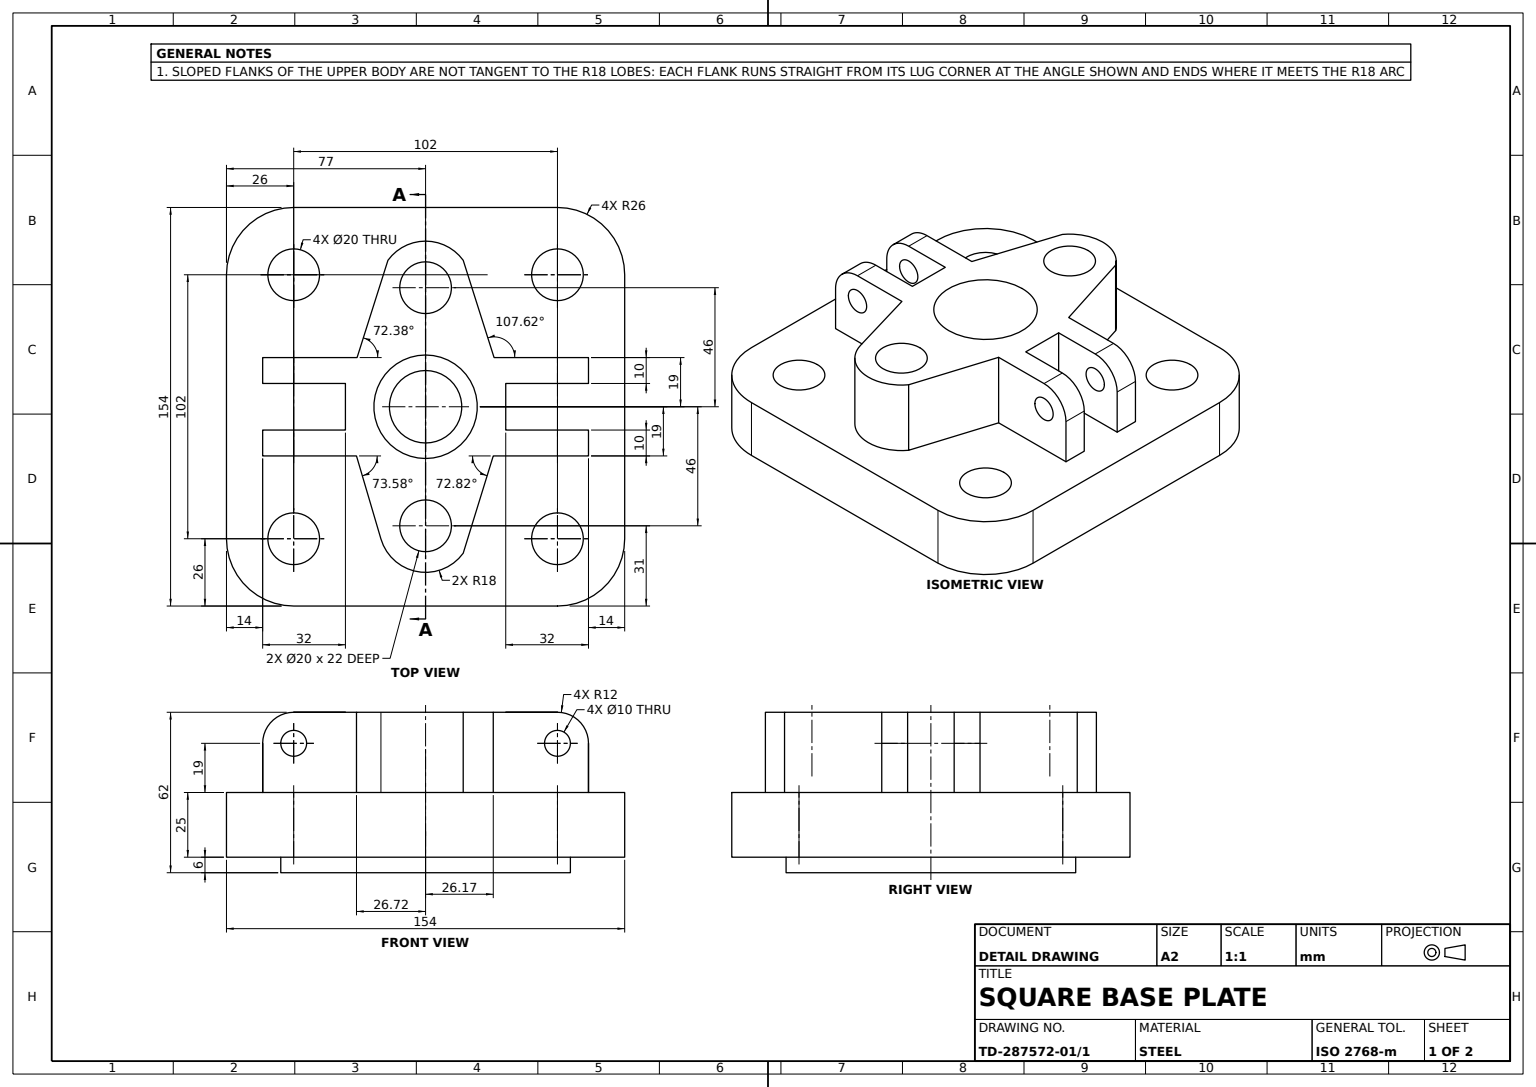
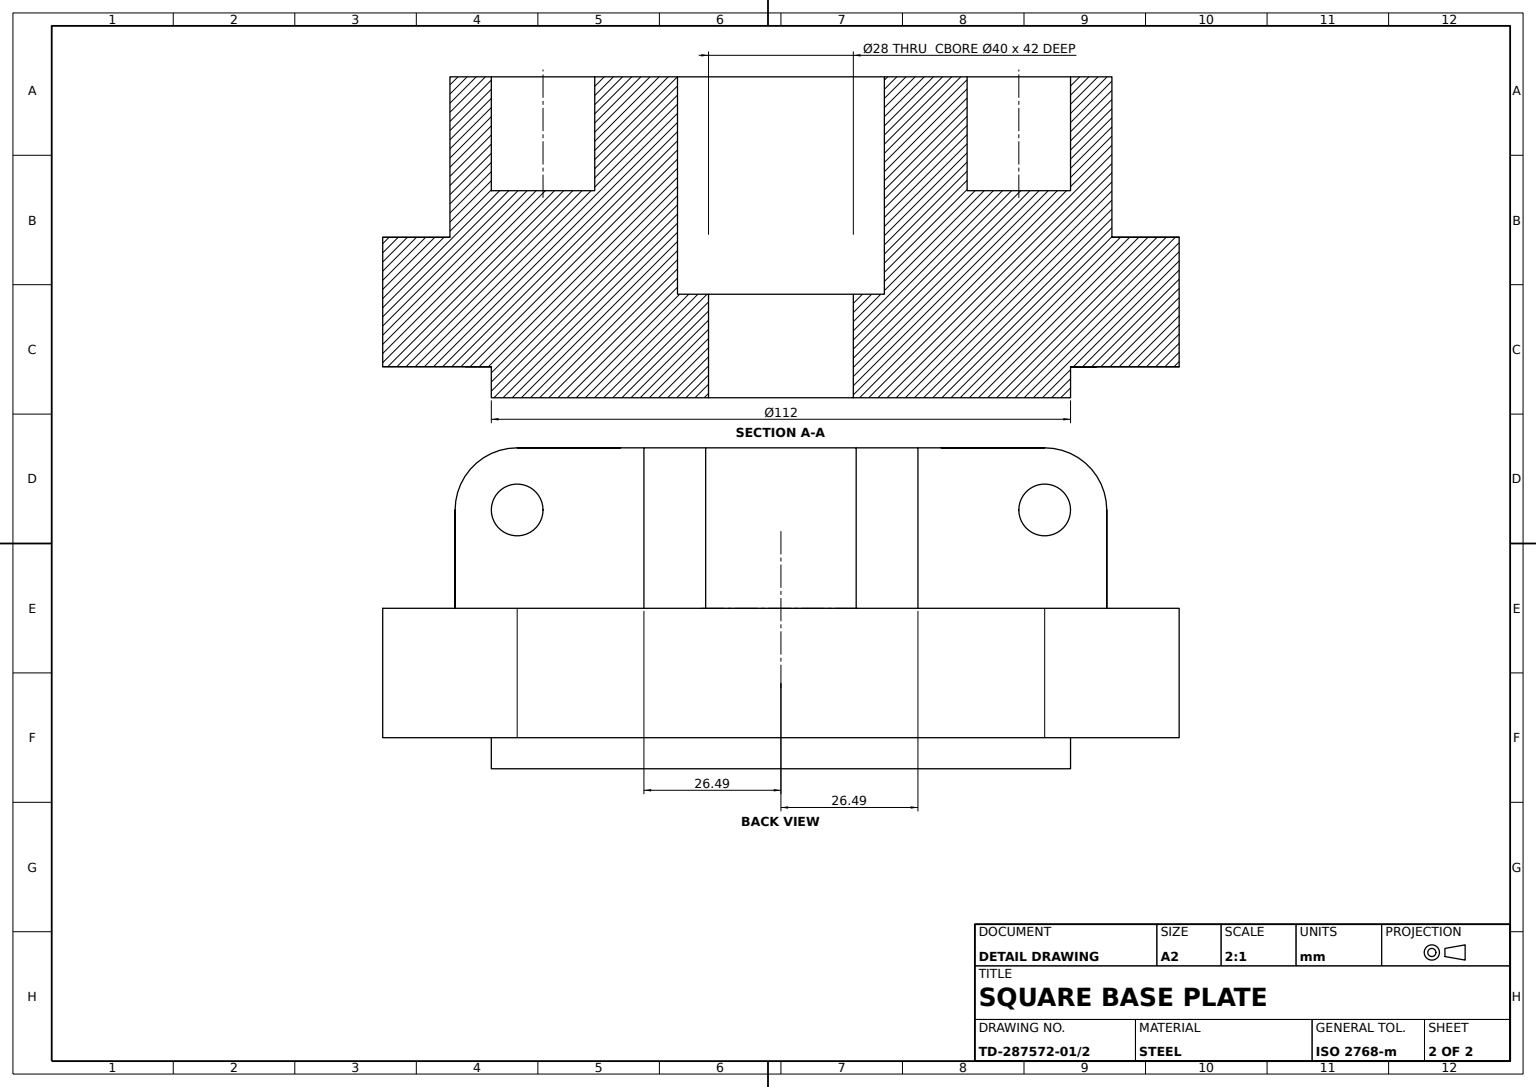
SolidWorks part; units mm, degrees
material "Plain Carbon Steel"
ref_plane "Front Plane" through (0, 0, 0) normal (0, 0, 1) x (1, 0, 0)
ref_plane "Top Plane" through (0, 0, 0) normal (0, 1, 0) x (1, 0, 0)
ref_plane "Right Plane" through (0, 0, 0) normal (1, 0, 0) x (0, 0, -1)
sketch "Base Plate Sketch" plane through (0, 0, 0) normal (0, 1, 0) x (1, 0, 0)
  line L1 (77, 0) -> (77, 51)
  line L2 (51, 77) -> (-51, 77)
  line L3 (-77, 51) -> (-77, -51)
  line L4 (-51, -77) -> (51, -77)
  line L5 (77, -51) -> (77, 0)
  arc A0 (51, -77) -> (77, -51) centre (51, -51) ccw
  arc A1 (-77, -51) -> (-51, -77) centre (-51, -51) ccw
  arc A2 (77, 51) -> (51, 77) centre (51, 51) ccw
  arc A3 (-51, 77) -> (-77, 51) centre (-51, 51) ccw
  point P11 (-77, -77)
  point P14 (77, 77)
  point P17 (-77, 77)
  dimension "D6" = 26
  dimension "D1" = 154
  dimension "D2" = 154
  dimension "D3" = 77
  dimension "D4" = 77
  dimension "D5" = 77
extrude "Base Plate" add sketch "Base Plate Sketch" along normal blind 25
sketch "Plate Mounting Holes Sketch" plane through (0, 25, 0) normal (0, 1, 0) x (1, 0, 0)
  circle A0 centre (-51, 51) radius 10
  circle A1 centre (51, 51) radius 10
  circle A2 centre (51, -51) radius 10
  circle A3 centre (-51, -51) radius 10
  dimension "D1" = 20
  dimension "D2" = 20
  dimension "D3" = 20
  dimension "D4" = 20
extrude "Plate Mounting Holes" cut sketch "Plate Mounting Holes Sketch" against normal blind 112
sketch "Central Boss Sketch" plane through (0, 25, 0) normal (0, 1, 0) x (1, 0, 0)
  line L2 (14.5512, 56.5954) -> (29.5457, 9.3837)
  line L3 (-14.5512, 56.5954) -> (-29.5457, 9.3837)
  line L4 (-29.7363, -8.7609) -> (-17.2662, -51.087)
  line L5 (14.5512, -56.5954) -> (30.6852, -4.4069)
  arc A1 (-17.2662, -51.087) -> (14.5512, -56.5954) centre (0, -46) ccw
  arc A2 (-29.5457, 9.3837) -> (-29.7363, -8.7609) centre (0, 0) ccw
  arc A3 (14.5512, 56.5954) -> (-14.5512, 56.5954) centre (0, 46) ccw
  arc A4 (30.6852, -4.4069) -> (29.5457, 9.3837) centre (0, 0) ccw
  dimension "D1" = 18
  dimension "D2" = 18
  dimension "D4" = 31
  dimension "D8" = 46
  dimension "D10" = 46
  dimension "D3" = 52.1886
  dimension "D5" = 47.2117
  dimension "D6" = 42.3261
  dimension "D7" = 47.2117
  dimension "D9" = 30.6178
  dimension "D11" = 178.796
extrude "Central Boss" add sketch "Central Boss Sketch" along normal blind 31
sketch "Lug Pair A Sketch" plane through (0, 56, 0) normal (0, 1, 0) x (1, 0, 0)
  line L0 (0, 0) -> (31, 0)
  line L1 (31, 9) -> (31, -9)
  line L2 (24.4949, -19) -> (63, -19)
  line L3 (63, -19) -> (63, -9)
  line L4 (63, -9) -> (31, -9)
  line L6 (63, 9) -> (31, 9)
  line L7 (31, -19) -> (26.1737, -19)
  line L8 (24.4949, 19) -> (63, 19)
  line L10 (31, 19) -> (63, 19)
  line L11 (63, 19) -> (63, 9)
  line L12 (14.5512, -56.5954) -> (30.6852, -4.4069) construction
  arc A0 (30.6852, -4.4069) -> (29.5457, 9.3837) centre (0, 0) ccw construction
  arc A1 (24.4949, -19) -> (24.4949, 19) centre (0, 0) ccw
  line M10 (14.5512, -56.5954) -> (30.6852, -4.4069)
  arc M11 (30.6852, -4.4069) -> (29.5457, 9.3837) centre (0, 0) ccw
  line M12 (29.5457, 9.3837) -> (14.5512, 56.5954)
  dimension "D1" = 9.9437
  dimension "D2" = 48.4488
  dimension "D3" = 47.5954
extrude "Lug Pair A" add sketch "Lug Pair A Sketch" against normal blind 31 contours L11 L8 L1 L6 M12 M11 | A1 L2 L3 L4 L1 M10 M11 | A1 L8 M12 | A1 L2 M10 | A1 M10
sketch "Lug Pair B Sketch" plane through (0, 56, 0) normal (0, 1, 0) x (1, 0, 0)
  line L0 (-77, 51) -> (-77, -51) construction
  line L1 (-31, 0) -> (-31, 9)
  line L2 (-24.4949, 19) -> (-63, 19)
  line L3 (-63, 19) -> (-63, 9)
  line L4 (-63, 9) -> (-31, 9)
  line L5 (-31, 0) -> (-31, -9)
  line L6 (-63, -9) -> (-31, -9)
  line L8 (-24.4949, -19) -> (-63, -19)
  line L9 (-63, -19) -> (-63, -9)
  arc A0 (-29.5457, 9.3837) -> (-29.7363, -8.7609) centre (0, 0) ccw construction
  arc A1 (-24.4949, 19) -> (-24.4949, -19) centre (0, 0) ccw
  line M14 (-14.5512, 56.5954) -> (-29.5457, 9.3837)
  arc M15 (-29.5457, 9.3837) -> (-29.7363, -8.7609) centre (0, 0) ccw
  line M16 (-29.7363, -8.7609) -> (-17.2662, -51.087)
  dimension "D1" = 19
  dimension "D2" = 19
  dimension "D3" = 14
  dimension "D4" = 14
  dimension "D5" = 10
  dimension "D6" = 18
extrude "Lug Pair B" add sketch "Lug Pair B Sketch" against normal blind 31 contours L9 L8 L5 L6 M16 M15 | L3 L4 L1 L2 M15 M14 | A1 L8 M16 | A1 L2 M14
sketch "Lug Pin Holes Sketch" plane through (0, 0, 19) normal (0, 0, 1) x (1, 0, 0)
  line L0 (26.1737, 25) -> (26.1737, 56) construction
  line L1 (26.1737, 25) -> (63, 25) construction
  circle A0 centre (51, 44) radius 5
  circle A1 centre (-51, 44) radius 5
  dimension "D1" = 10
  dimension "D2" = 24.8263
  dimension "D3" = 77.1737
  dimension "D4" = 19
extrude "Lug Pin Holes" cut sketch "Lug Pin Holes Sketch" against normal blind 118
fillet "Lug A Fillet 1" radius 12 1 edges at (63, 56, 14)
fillet "Lug A Fillet 2" radius 12 1 edges at (63, 56, -14)
fillet "Lug B Fillet 1" radius 12 1 edges at (-63, 56, -14)
fillet "Lug B Fillet 2" radius 12 1 edges at (-63, 56, 14)
sketch "Central Bore Sketch" plane through (0, 56, 0) normal (0, 1, 0) x (1, 0, 0)
  circle A0 centre (0, 0) radius 14
  dimension "D1" = 28
extrude "Central Bore" cut sketch "Central Bore Sketch" against normal blind 118
sketch "Bore Counterbore Sketch" plane through (0, 56, 0) normal (0, 1, 0) x (1, 0, 0)
  circle A0 centre (0, 0) radius 20
  dimension "D1" = 40
extrude "Bore Counterbore" cut sketch "Bore Counterbore Sketch" against normal blind 42
sketch "Bottom Spigot Sketch" plane through (0, 0, 0) normal (0, -1, 0) x (1, 0, 0)
  circle A0 centre (0, 0) radius 56
  dimension "D1" = 112
extrude "Bottom Spigot" add sketch "Bottom Spigot Sketch" along normal blind 6
sketch "Spigot Bore Sketch" plane through (0, 0, 0) normal (0, 1, 0) x (1, 0, 0)
  circle A0 centre (0, 0) radius 14
  dimension "D1" = 28
extrude "Spigot Bore" cut sketch "Spigot Bore Sketch" against normal blind 120
sketch "Flange Hole 1 Sketch" plane through (0, 56, 0) normal (0, 1, 0) x (1, 0, 0)
  circle A0 centre (0, 46) radius 10
  dimension "D1" = 20
extrude "Flange Hole 1" cut sketch "Flange Hole 1 Sketch" against normal blind 22
sketch "Flange Hole 2 Sketch" plane through (0, 56, 0) normal (0, 1, 0) x (1, 0, 0)
  circle A0 centre (0, -46) radius 10
  dimension "D1" = 20
extrude "Flange Hole 2" cut sketch "Flange Hole 2 Sketch" against normal blind 22
